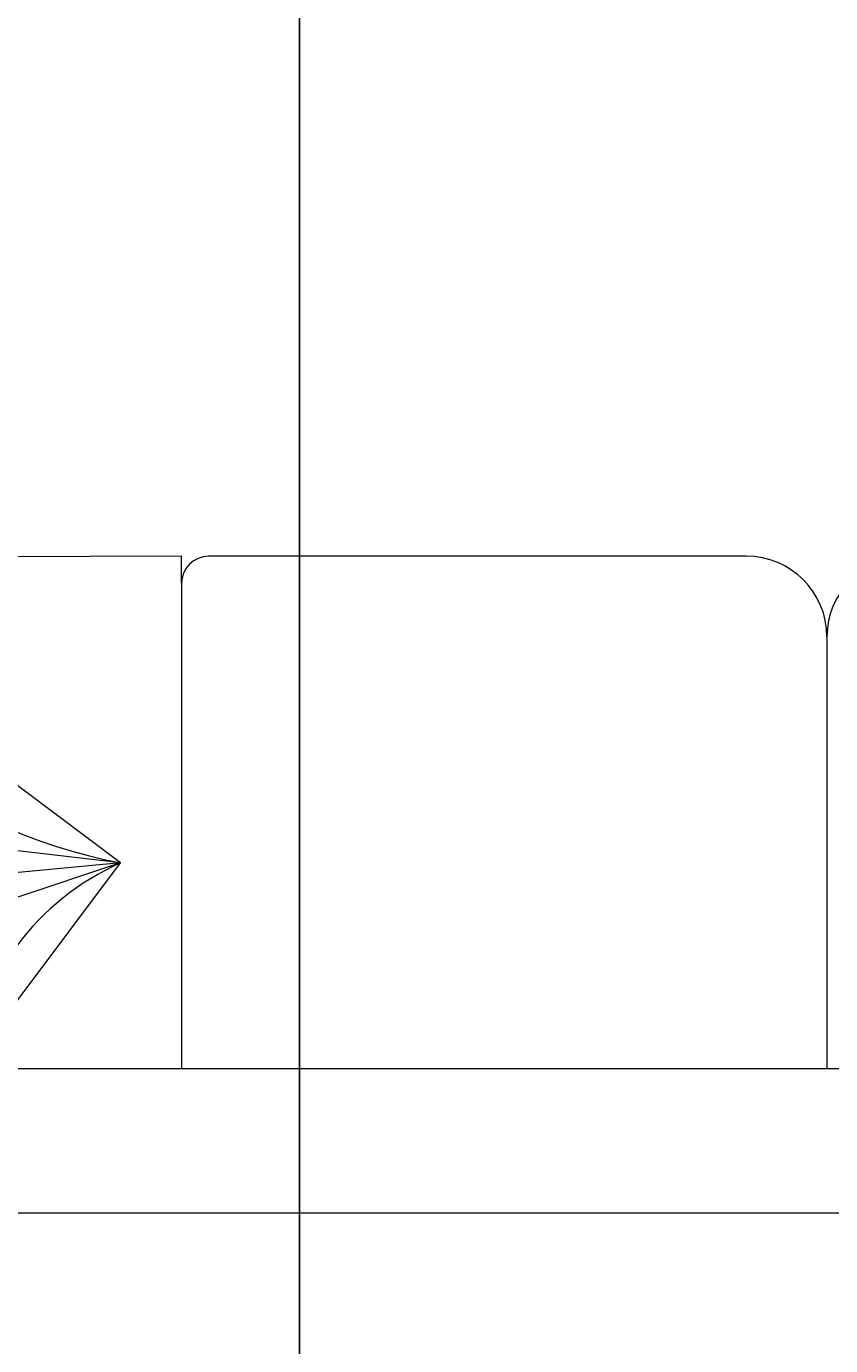
# Model space of a CAD drawing. Units: inches. Extents: x -61 to 1599, y -1316 to 257.
# Tile 106 of 204: x 170 to 200, y -166 to -117. Entities that reach past the tile are written whole.
import ezdxf

# ---------------------------------------------------------------- set-up
doc = ezdxf.new("R2010")
doc.units = ezdxf.units.IN
doc.header["$MEASUREMENT"] = 0
doc.layers.add('A-ANNO-DIMS', color=2, linetype='Continuous', lineweight=18)
doc.layers.add('FURNITURE', color=83, linetype='Continuous', lineweight=18)
doc.styles.get("Standard").update_dxf_attribs({"font": 'arial.ttf'})
doc.dimstyles.get("Standard").update_dxf_attribs({"dimtxt": 0.18, "dimasz": 0.18, "dimexe": 0.18, "dimexo": 0.0625, "dimgap": 0.09, "dimtad": 0, "dimtih": 1, "dimtoh": 1, "dimdec": 0, "dimzin": 0, "dimdsep": 46, "dimlunit": 3, "dimtxsty": 'Standard', "dimcen": 0.09, "dimadec": 0, "dimazin": 0, "dimtfac": 1, "dimtdec": 0, "dimtofl": 0, "dimtmove": 0, "dimatfit": 3, "dimfxl": 1, "dimtolj": 1, "dimtzin": 0, "dimarcsym": 0})

# ---------------------------------------------------------------- blocks, each defined once
blk = doc.blocks.new('SOFA-THREE-SEAT')
for p, q in [((30, 24.442), (6.996, 24.38)), ((30, 23.442), (29.997, 24.442)), ((51, 24.442), (31, 24.442)), ((30, 23.442), (30, 5.382)), ((54, 21.442), (54, 5.382)), ((54, 21.442), (54, 21.442)), ((27.729, 13.028), (23.263, 13.551)), ((27.729, 13.028), (21.735, 12.472)), ((27.729, 13.028), (23.795, 11.722))]:
    blk.add_line(p, q)
blk.add_lwpolyline([(78, 8.382), (78, 23, -0.414214), (81, 26), (81, 26, -0.414214), (84, 23), (84, 3, -0.414214), (81, 0), (3, 0, -0.414214), (0, 3), (0, 23, -0.414214), (3, 26), (3, 26, -0.414214), (6, 23), (6, 8.382, 0.414214), (9, 5.382), (75, 5.382, 0.414214)], format="xyb", close=True)
blk.add_lwpolyline([(27.729, 13.028), (12.664, 24.333), (6.926, 16.687), (21.991, 5.382)], close=True)
for centre, radius, start, end in [((31.951, 34.345), 21.731, 207.4316, 258.7956), ((31, 23.442), 1, 90, 180), ((51, 21.442), 3, 360, 90), ((57, 21.442), 3, 90, 180), ((31.717, 4.059), 9.816, 113.9742, 172.253)]:
    blk.add_arc(centre, radius, start, end)
blk = doc.blocks.new('*D670')
at = {"layer": 'A-ANNO-DIMS', "color": 0, "lineweight": -2, "transparency": 16777216}
for p, q in [((145.375, -161.442), (145.375, -174.159)), ((229.375, -161.442), (229.375, -174.159)), ((145.555, -173.979), (186.47, -173.979)), ((229.195, -173.979), (188.279, -173.979))]:
    blk.add_line(p, q, dxfattribs=at)
at = {"layer": 'A-ANNO-DIMS', "color": 0, "transparency": 16777216}
for points in [[(145.555, -173.949), (145.555, -174.009), (145.375, -173.979)], [(229.195, -173.949), (229.195, -174.009), (229.375, -173.979)]]:
    blk.add_solid(points, dxfattribs=at)
at = {"layer": 'DEFPOINTS', "color": 0, "transparency": 16777216}
for p in [(145.375, -161.379), (229.375, -161.379), (229.375, -173.979)]:
    blk.add_point(p, dxfattribs=at)
at = {"layer": 'A-ANNO-DIMS', "color": 0, "transparency": 16777216, "insert": (187.375, -173.979), "char_height": 0.18, "attachment_point": 5}
blk.add_mtext('\\A1;SOFA 84 TYP.', dxfattribs=at)
blk = doc.blocks.new('*D687')
at = {"layer": 'A-ANNO-DIMS', "color": 0, "lineweight": -2, "transparency": 16777216}
for p, q in [((289.418, 181.677), (-61.077, 181.677)), ((-60.897, 181.497), (-60.897, -528.952)), ((-60.897, -1239.765), (-60.897, -529.316)), ((319.64, -1239.945), (-61.077, -1239.945))]:
    blk.add_line(p, q, dxfattribs=at)
at = {"layer": 'A-ANNO-DIMS', "color": 0, "transparency": 16777216}
for points in [[(-60.927, 181.497), (-60.867, 181.497), (-60.897, 181.677)], [(-60.927, -1239.765), (-60.867, -1239.765), (-60.897, -1239.945)]]:
    blk.add_solid(points, dxfattribs=at)
at = {"layer": 'DEFPOINTS', "color": 0, "transparency": 16777216}
for p in [(289.481, 181.677), (-60.897, -1239.945), (319.703, -1239.945)]:
    blk.add_point(p, dxfattribs=at)
at = {"layer": 'A-ANNO-DIMS', "color": 0, "transparency": 16777216, "insert": (-60.897, -529.134), "char_height": 0.18, "attachment_point": 5}
blk.add_mtext('\\A1;1421.6', dxfattribs=at)
blk = doc.blocks.new('*D700')
at = {"layer": 'A-ANNO-DIMS', "color": 0, "lineweight": -2, "transparency": 16777216}
for p, q in [((14.703, -616.882), (14.703, 257.457)), ((14.883, 257.277), (96.772, 257.277)), ((179.572, 257.277), (97.683, 257.277)), ((179.752, -616.882), (179.752, 257.457))]:
    blk.add_line(p, q, dxfattribs=at)
at = {"layer": 'A-ANNO-DIMS', "color": 0, "transparency": 16777216}
for points in [[(14.883, 257.307), (14.883, 257.247), (14.703, 257.277)], [(179.572, 257.307), (179.572, 257.247), (179.752, 257.277)]]:
    blk.add_solid(points, dxfattribs=at)
at = {"layer": 'DEFPOINTS', "color": 0, "transparency": 16777216}
for p in [(179.752, 257.277), (14.703, -616.945), (179.752, -616.945)]:
    blk.add_point(p, dxfattribs=at)
at = {"layer": 'A-ANNO-DIMS', "color": 0, "transparency": 16777216, "insert": (97.227, 257.277), "char_height": 0.18, "attachment_point": 5}
blk.add_mtext('\\A1;165.05', dxfattribs=at)

msp = doc.modelspace()

# ---------------------------------------------------------------- block references
at = {"layer": 'FURNITURE'}
msp.add_blockref('SOFA-THREE-SEAT', (145.375, -161.379), dxfattribs=at)

# ---------------------------------------------------------------- dimensions: what is measured, and where the dimension line sits
at = {"layer": 'A-ANNO-DIMS'}
dim = msp.add_linear_dim(base=(179.7521, 257.2771), p1=(14.7028, -616.9446), p2=(179.7521, -616.9446), dimstyle='Standard', override={"dimdec": 2, "dimlfac": 1, "dimrnd": 0, "dimzin": 0, "dimdsep": 46, "dimlunit": 2}, dxfattribs=at)
dim.commit()
dim.dimension.update_dxf_attribs({"geometry": '*D700', "text_midpoint": (97.2274, 257.2771)})
dim = msp.add_linear_dim(base=(-60.8972, -1239.9446), p1=(289.4807, 181.6771), p2=(319.7028, -1239.9446), angle=90, dimstyle='Standard', override={"dimdec": 1, "dimlfac": 1, "dimrnd": 0, "dimzin": 0, "dimdsep": 46, "dimlunit": 2}, dxfattribs=at)
dim.commit()
dim.dimension.update_dxf_attribs({"geometry": '*D687', "text_midpoint": (-60.8972, -529.1337)})
dim = msp.add_linear_dim(base=(229.3746, -173.9792), p1=(145.3746, -161.3792), p2=(229.3746, -161.3792), text='SOFA <> TYP.', dimstyle='Standard', override={"dimdec": 0, "dimlfac": 1, "dimrnd": 0, "dimzin": 0, "dimdsep": 46, "dimlunit": 2}, dxfattribs=at)
dim.commit()
dim.dimension.update_dxf_attribs({"geometry": '*D670', "text_midpoint": (187.3746, -173.9792)})

doc.saveas('drawing.dxf')
